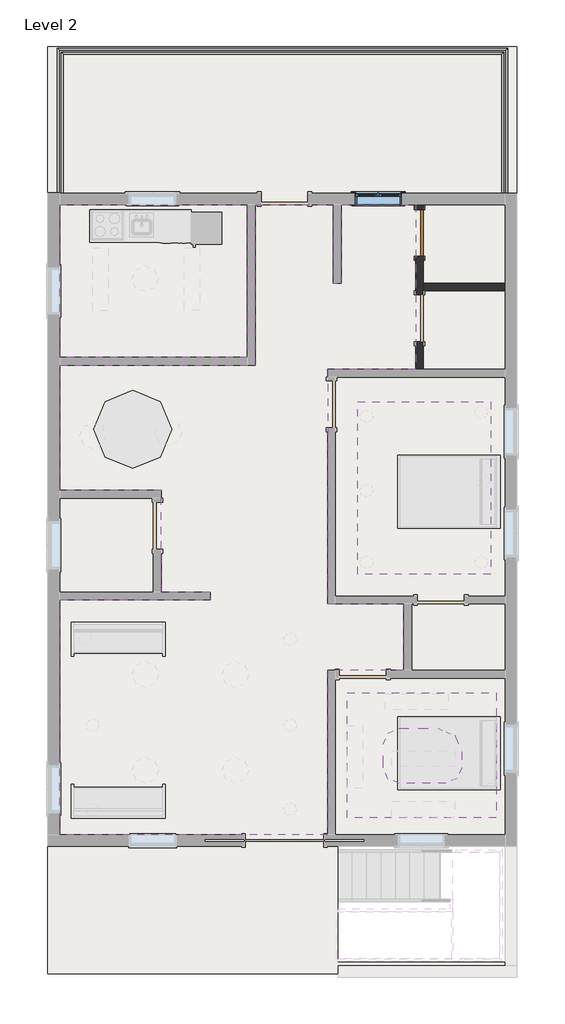
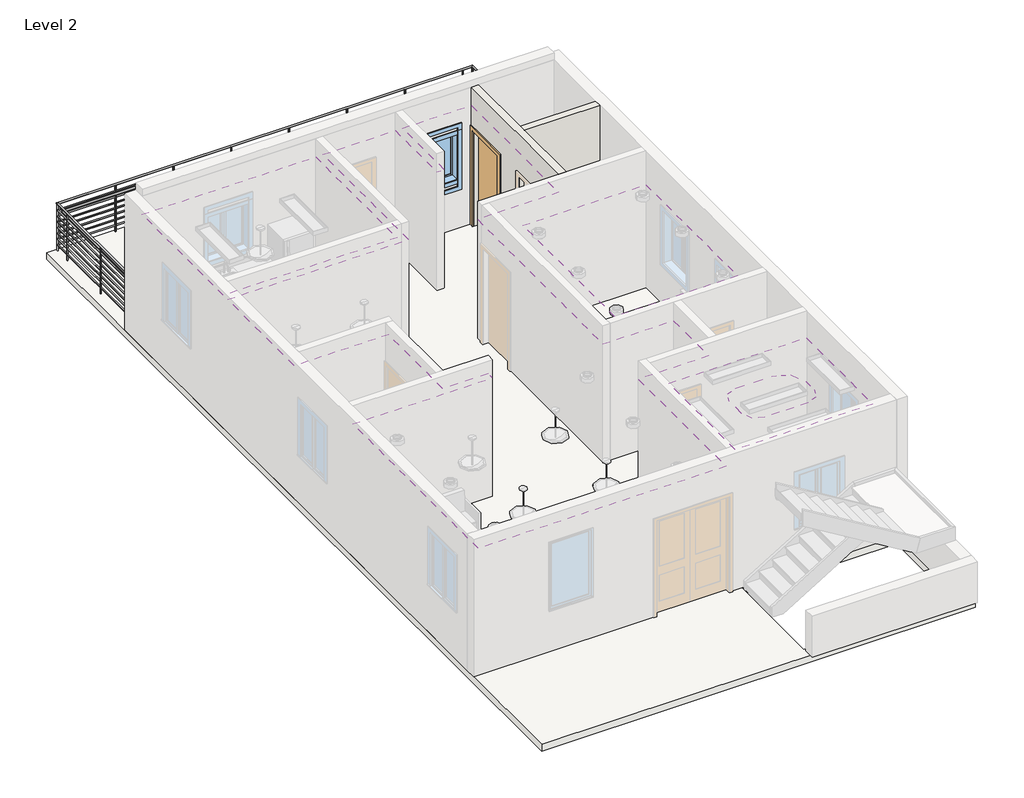
# One storey, part 2 of 3: 7 coverings, 2 walls, 2 windows, 1 door, 1 railing, 1 slab.
"""IFC4 building model written with IfcOpenShell, lengths in millimetres."""

from ifc_helpers import new_model, si_unit, point, frame, frame_2d, origin, place, context, project, spatial, polyline, circle_curve, ellipse_curve, trimmed, segment, composite_curve, outline, extrude, faceted_brep, transform, mapped, element, save
from ifc_brep_helpers import plane_surface, cylinder_surface, advanced_brep
from components import single_flush_single_door_686f89d2, window_419b5846

model = new_model("IFC4")

# Units and contexts
model_context = context("Model", 3, world=origin())
ifc_project = project(units=[si_unit("LENGTHUNIT", "METRE", prefix="MILLI")], contexts=[model_context])

# Site, building, storey
site = spatial("IfcSite", under=ifc_project)
building = spatial("IfcBuilding", under=site)
storey = spatial("IfcBuildingStorey", under=building, Name="Level 2", Elevation=3200.4)

# Coverings
placement = place(None, origin())
element("IfcCovering", 1, ObjectType="design", at=placement, inside=storey, context=model_context, shape_type="SweptSolid", body=[
    extrude(outline(polyline([(-1441.8942717, 10130.0102367), (-1441.8942717, 6777.2102367), (-4032.6942717, 6777.2102367), (-4032.6942717, 10130.0102367), (-1441.8942717, 10130.0102367)]), holes=[composite_curve([segment(polyline([(-1961.8324971, 9831.2802454), (-3524.6942717, 9831.2802454)]), True, "CONTINUOUS"), segment(trimmed(circle_curve(frame_2d((-3524.6942717, 9628.0802454)), 203.2), [point((-3524.6942717, 9831.2802454))], [point((-3727.8942717, 9628.0802454))], True, "CARTESIAN"), True, "CONTINUOUS"), segment(polyline([(-3727.8942717, 9628.0802454), (-3727.8942717, 7367.4802454)]), True, "CONTINUOUS"), segment(trimmed(circle_curve(frame_2d((-3397.6942717, 7367.4802454)), 330.2), [point((-3727.8942717, 7367.4802454))], [point((-3397.6942717, 7037.2802454))], True, "CARTESIAN"), True, "CONTINUOUS"), segment(polyline([(-3397.6942717, 7037.2802454), (-2178.4942717, 7037.2802454)]), True, "CONTINUOUS"), segment(trimmed(circle_curve(frame_2d((-2178.4942717, 7469.0802454)), 431.8), [point((-2178.4942717, 7037.2802454))], [point((-1746.6942717, 7469.0802454))], True, "CARTESIAN"), True, "CONTINUOUS"), segment(polyline([(-1746.6942717, 7469.0802454), (-1746.6942717, 9616.14202)]), True, "CONTINUOUS"), segment(trimmed(circle_curve(frame_2d((-1961.8324971, 9616.14202)), 215.1382254), [point((-1746.6942717, 9616.14202))], [point((-1961.8324971, 9831.2802454))], True, "CARTESIAN"), True, "CONTINUOUS")], self_intersect=False)]), frame((0.0, 0.0, 5892.8), z_axis=(0.0, 0.0, 1.0), x_axis=(1.0, 0.0, 0.0)), (0.0, 0.0, 1.0), 50.8),
])
element("IfcCovering", 2, ObjectType="design", at=placement, inside=storey, context=model_context, shape_type="SweptSolid", body=[
    extrude(outline(polyline([(-1336.1469547, 4466.8667258), (-1336.1469547, 2028.4667258), (-4231.7469547, 2028.4667258), (-4231.7469547, 4466.8667258), (-1336.1469547, 4466.8667258)]), holes=[polyline([(-1663.4737397, 4144.2687658), (-3949.4737397, 4144.2687658), (-3949.4737397, 2315.4687658), (-1663.4737397, 2315.4687658), (-1663.4737397, 4144.2687658)])]), frame((0.0, 0.0, 5880.0205268), z_axis=(0.0, 0.0, 1.0), x_axis=(1.0, 0.0, 0.0)), (0.0, 0.0, 1.0), 50.8),
])
element("IfcCovering", 3, ObjectType="inner", at=placement, inside=storey, context=model_context, shape_type="SweptSolid", body=[
    extrude(outline(composite_curve([segment(trimmed(circle_curve(frame_2d((-2465.984708, 3312.1230358)), 457.2), [point((-2465.984708, 3769.3230358))], [point((-2008.784708, 3312.1230358))], False, "CARTESIAN"), True, "CONTINUOUS"), segment(polyline([(-2008.784708, 3312.1230358), (-2008.784708, 3007.3230358)]), True, "CONTINUOUS"), segment(trimmed(circle_curve(frame_2d((-2313.584708, 3007.3230358)), 304.8), [point((-2008.784708, 3007.3230358))], [point((-2313.584708, 2702.5230358))], False, "CARTESIAN"), True, "CONTINUOUS"), segment(polyline([(-2313.584708, 2702.5230358), (-3227.984708, 2702.5230358)]), True, "CONTINUOUS"), segment(trimmed(circle_curve(frame_2d((-3227.984708, 3007.3230358)), 304.8), [point((-3227.984708, 2702.5230358))], [point((-3532.784708, 3007.3230358))], False, "CARTESIAN"), True, "CONTINUOUS"), segment(polyline([(-3532.784708, 3007.3230358), (-3532.784708, 3464.5230358)]), True, "CONTINUOUS"), segment(trimmed(circle_curve(frame_2d((-3227.984708, 3464.5230358)), 304.8), [point((-3532.784708, 3464.5230358))], [point((-3227.984708, 3769.3230358))], False, "CARTESIAN"), True, "CONTINUOUS"), segment(polyline([(-3227.984708, 3769.3230358), (-2465.984708, 3769.3230358)]), True, "CONTINUOUS")], self_intersect=False)), frame((0.0, 0.0, 5842.0), z_axis=(0.0, 0.0, 1.0), x_axis=(1.0, 0.0, 0.0)), (0.0, 0.0, 1.0), 50.8),
])
element("IfcCovering", 4, ObjectType="inner", at=placement, inside=storey, context=model_context, shape_type="SweptSolid", body=[
    extrude(outline(polyline([(-4619.1572065, 4901.2206867), (-4619.1572065, 1700.8206867), (-9838.8572065, 1700.8206867), (-9838.8572065, 6272.8206867), (-6905.1572065, 6272.8206867), (-6905.1572065, 6425.2206867), (-7857.6572065, 6425.2206867), (-7857.6572065, 8406.4206867), (-9838.8572065, 8406.4206867), (-9838.8572065, 10844.8206867), (-6028.8572065, 10844.8206867), (-6028.8572065, 13969.0206867), (-4504.8572065, 13969.0206867), (-4504.8572065, 12445.0206867), (-4352.4572065, 12445.0206867), (-4352.4572065, 13969.0206867), (-2904.6572065, 13969.0206867), (-2904.6572065, 10768.6206867), (-4619.1572065, 10768.6206867), (-4619.1572065, 6196.6206867), (-3133.2572065, 6196.6206867), (-3133.2572065, 4901.2206867), (-4619.1572065, 4901.2206867)])), frame((0.0, 0.0, 5842.0), z_axis=(0.0, 0.0, 1.0), x_axis=(1.0, 0.0, 0.0)), (0.0, 0.0, 1.0), 50.8),
])
element("IfcCovering", 5, ObjectType="inner", at=placement, inside=storey, context=model_context, shape_type="SweptSolid", body=[
    extrude(outline(polyline([(-4619.1572065, 4901.2206867), (-4619.1572065, 1700.8206867), (-9838.8572065, 1700.8206867), (-9838.8572065, 6272.8206867), (-6905.1572065, 6272.8206867), (-6905.1572065, 6425.2206867), (-7857.6572065, 6425.2206867), (-7857.6572065, 8406.4206867), (-9838.8572065, 8406.4206867), (-9838.8572065, 10844.8206867), (-6028.8572065, 10844.8206867), (-6028.8572065, 13969.0206867), (-4504.8572065, 13969.0206867), (-4504.8572065, 12445.0206867), (-4352.4572065, 12445.0206867), (-4352.4572065, 13969.0206867), (-2904.6572065, 13969.0206867), (-2904.6572065, 10768.6206867), (-4619.1572065, 10768.6206867), (-4619.1572065, 6196.6206867), (-3133.2572065, 6196.6206867), (-3133.2572065, 4901.2206867), (-4619.1572065, 4901.2206867)])), frame((0.0, 0.0, 5842.0), z_axis=(0.0, 0.0, 1.0), x_axis=(1.0, 0.0, 0.0)), (0.0, 0.0, 1.0), 50.8),
])
element("IfcCovering", 6, ObjectType="inner", at=placement, inside=storey, context=model_context, shape_type="SweptSolid", body=[
    extrude(outline(polyline([(-9838.8572065, 13969.0206867), (-6181.2572065, 13969.0206867), (-6181.2572065, 10997.2206867), (-9838.8572065, 10997.2206867), (-9838.8572065, 13969.0206867)])), frame((0.0, 0.0, 5842.0), z_axis=(0.0, 0.0, 1.0), x_axis=(1.0, 0.0, 0.0)), (0.0, 0.0, 1.0), 50.8),
])
element("IfcCovering", 7, ObjectType="inner", at=placement, inside=storey, context=model_context, shape_type="SweptSolid", body=[
    extrude(outline(polyline([(-9838.8572065, 13969.0206867), (-6181.2572065, 13969.0206867), (-6181.2572065, 10997.2206867), (-9838.8572065, 10997.2206867), (-9838.8572065, 13969.0206867)])), frame((0.0, 0.0, 5842.0), z_axis=(0.0, 0.0, 1.0), x_axis=(1.0, 0.0, 0.0)), (0.0, 0.0, 1.0), 50.8),
])

# Door
single_flush_single_door_shape = single_flush_single_door_686f89d2(model_context)
element("IfcDoor", 8, ObjectType="Single-Flush : single door", at=placement, inside=storey, context=model_context, shape_type="MappedRepresentation", body=[
    mapped(single_flush_single_door_shape, transform((-2828.4572065, 13422.9206867, 3200.4), x_axis=(0.0, 1.0, 0.0), y_axis=(-1.0, 0.0, 0.0), z_axis=(0.0, 0.0, 1.0))),
])

# Railing
element("IfcRailing", 9, ObjectType="Guardrail - Pipe", at=placement, inside=storey, context=model_context, shape_type="SolidModel", body=[
    advanced_brep(
    [(-9769.0072065, 14210.3206867, 4095.75), (-9807.1072065, 14210.3206867, 4095.75), (-9769.0072065, 16909.0706867, 4095.75), (-9807.1072065, 16947.1706867, 4095.75), (-1221.9072065, 16909.0706867, 4095.75), (-1183.8072065, 16947.1706867, 4095.75), (-1221.9072065, 14210.3206867, 4095.75), (-1183.8072065, 14210.3206867, 4095.75)],
    [
        (0, 1, circle_curve(frame((-9788.0572065, 14210.3206867, 4095.75), z_axis=(0.0, -1.0, 0.0), x_axis=(-1.0, 0.0, 0.0)), 19.05)),
        (1, 0, circle_curve(frame((-9788.0572065, 14210.3206867, 4095.75), z_axis=(0.0, -1.0, 0.0), x_axis=(-1.0, 0.0, 0.0)), 19.05)),
        (0, 2),
        (2, 3, ellipse_curve(frame((-9788.0572065, 16928.1206867, 4095.75), z_axis=(-0.7071067811865475, -0.7071067811865475, 0.0), x_axis=(0.7071067811865474, -0.7071067811865476, 0.0)), 26.9407684, 19.05)),
        (3, 1),
        (3, 2, ellipse_curve(frame((-9788.0572065, 16928.1206867, 4095.75), z_axis=(-0.7071067811865475, -0.7071067811865475, 0.0), x_axis=(0.7071067811865474, -0.7071067811865476, 0.0)), 26.9407684, 19.05)),
        (2, 4),
        (4, 5, ellipse_curve(frame((-1202.8572065, 16928.1206867, 4095.75), z_axis=(-0.7071067811865475, 0.7071067811865475, 0.0), x_axis=(-0.7071067811865476, -0.7071067811865474, 0.0)), 26.9407684, 19.05)),
        (5, 3),
        (5, 4, ellipse_curve(frame((-1202.8572065, 16928.1206867, 4095.75), z_axis=(-0.7071067811865475, 0.7071067811865475, 0.0), x_axis=(-0.7071067811865476, -0.7071067811865474, 0.0)), 26.9407684, 19.05)),
        (6, 7, circle_curve(frame((-1202.8572065, 14210.3206867, 4095.75), z_axis=(0.0, -1.0, 0.0), x_axis=(1.0, 0.0, 0.0)), 19.05)),
        (7, 6, circle_curve(frame((-1202.8572065, 14210.3206867, 4095.75), z_axis=(0.0, -1.0, 0.0), x_axis=(1.0, 0.0, 0.0)), 19.05)),
        (4, 6),
        (7, 5),
    ],
    [
        plane_surface(frame((-9788.0572065, 14210.3206867, 4114.8), z_axis=(0.0, -1.0, 0.0), x_axis=(0.0, 0.0, 1.0))),
        cylinder_surface(frame((-9788.0572065, 14210.3206867, 4095.75), z_axis=(0.0, -1.0, 0.0), x_axis=(-1.0, 0.0, 0.0)), 19.05),
        cylinder_surface(frame((-9788.0572065, 16928.1206867, 4095.75), z_axis=(-1.0, 0.0, 0.0), x_axis=(0.0, 1.0, 0.0)), 19.05),
        plane_surface(frame((-1202.8572065, 14210.3206867, 4114.8), z_axis=(0.0, -1.0, 0.0), x_axis=(0.0, 0.0, -1.0))),
        cylinder_surface(frame((-1202.8572065, 16928.1206867, 4095.75), z_axis=(0.0, 1.0, 0.0), x_axis=(1.0, 0.0, 0.0)), 19.05),
    ],
    [
        (0, [[1, 2]]),
        (1, [[-1, 3, 4, 5]]),
        (1, [[-2, -5, 6, -3]]),
        (2, [[-4, 7, 8, 9]]),
        (2, [[-6, -9, 10, -7]]),
        (3, [[11, 12]]),
        (4, [[-8, 13, -12, 14]]),
        (4, [[-10, -14, -11, -13]]),
    ],
),
    advanced_brep(
    [(-9845.2072065, 14210.3206867, 4248.15), (-9883.3072065, 14210.3206867, 4248.15), (-9845.2072065, 16985.2706867, 4248.15), (-9883.3072065, 17023.3706867, 4248.15), (-1145.7072065, 16985.2706867, 4248.15), (-1107.6072065, 17023.3706867, 4248.15), (-1145.7072065, 14210.3206867, 4248.15), (-1107.6072065, 14210.3206867, 4248.15)],
    [
        (0, 1, circle_curve(frame((-9864.2572065, 14210.3206867, 4248.15), z_axis=(0.0, -1.0, 0.0), x_axis=(-1.0, 0.0, 0.0)), 19.05)),
        (1, 0, circle_curve(frame((-9864.2572065, 14210.3206867, 4248.15), z_axis=(0.0, -1.0, 0.0), x_axis=(-1.0, 0.0, 0.0)), 19.05)),
        (0, 2),
        (2, 3, ellipse_curve(frame((-9864.2572065, 17004.3206867, 4248.15), z_axis=(-0.7071067811865475, -0.7071067811865475, 0.0), x_axis=(0.7071067811865474, -0.7071067811865476, 0.0)), 26.9407684, 19.05)),
        (3, 1),
        (3, 2, ellipse_curve(frame((-9864.2572065, 17004.3206867, 4248.15), z_axis=(-0.7071067811865475, -0.7071067811865475, 0.0), x_axis=(0.7071067811865474, -0.7071067811865476, 0.0)), 26.9407684, 19.05)),
        (2, 4),
        (4, 5, ellipse_curve(frame((-1126.6572065, 17004.3206867, 4248.15), z_axis=(-0.7071067811865475, 0.7071067811865475, 0.0), x_axis=(-0.7071067811865476, -0.7071067811865474, 0.0)), 26.9407684, 19.05)),
        (5, 3),
        (5, 4, ellipse_curve(frame((-1126.6572065, 17004.3206867, 4248.15), z_axis=(-0.7071067811865475, 0.7071067811865475, 0.0), x_axis=(-0.7071067811865476, -0.7071067811865474, 0.0)), 26.9407684, 19.05)),
        (6, 7, circle_curve(frame((-1126.6572065, 14210.3206867, 4248.15), z_axis=(0.0, -1.0, 0.0), x_axis=(1.0, 0.0, 0.0)), 19.05)),
        (7, 6, circle_curve(frame((-1126.6572065, 14210.3206867, 4248.15), z_axis=(0.0, -1.0, 0.0), x_axis=(1.0, 0.0, 0.0)), 19.05)),
        (4, 6),
        (7, 5),
    ],
    [
        plane_surface(frame((-9864.2572065, 14210.3206867, 4267.2), z_axis=(0.0, -1.0, 0.0), x_axis=(0.0, 0.0, 1.0))),
        cylinder_surface(frame((-9864.2572065, 14210.3206867, 4248.15), z_axis=(0.0, -1.0, 0.0), x_axis=(-1.0, 0.0, 0.0)), 19.05),
        cylinder_surface(frame((-9864.2572065, 17004.3206867, 4248.15), z_axis=(-1.0, 0.0, 0.0), x_axis=(0.0, 1.0, 0.0)), 19.05),
        plane_surface(frame((-1126.6572065, 14210.3206867, 4267.2), z_axis=(0.0, -1.0, 0.0), x_axis=(0.0, 0.0, -1.0))),
        cylinder_surface(frame((-1126.6572065, 17004.3206867, 4248.15), z_axis=(0.0, 1.0, 0.0), x_axis=(1.0, 0.0, 0.0)), 19.05),
    ],
    [
        (0, [[1, 2]]),
        (1, [[-1, 3, 4, 5]]),
        (1, [[-2, -5, 6, -3]]),
        (2, [[-4, 7, 8, 9]]),
        (2, [[-6, -9, 10, -7]]),
        (3, [[11, 12]]),
        (4, [[-8, 13, -12, 14]]),
        (4, [[-10, -14, -11, -13]]),
    ],
),
    advanced_brep(
    [(-9851.5572065, 14210.3206867, 4102.1), (-9876.9572065, 14210.3206867, 4102.1), (-9876.9572065, 17017.0206867, 4102.1), (-9851.5572065, 16991.6206867, 4102.1), (-1113.9572065, 17017.0206867, 4102.1), (-1139.3572065, 16991.6206867, 4102.1), (-1139.3572065, 14210.3206867, 4102.1), (-1113.9572065, 14210.3206867, 4102.1)],
    [
        (0, 1, circle_curve(frame((-9864.2572065, 14210.3206867, 4102.1), z_axis=(0.0, -1.0, 0.0), x_axis=(-1.0, 0.0, 0.0)), 12.7)),
        (1, 0, circle_curve(frame((-9864.2572065, 14210.3206867, 4102.1), z_axis=(0.0, -1.0, 0.0), x_axis=(-1.0, 0.0, 0.0)), 12.7)),
        (1, 2),
        (2, 3, ellipse_curve(frame((-9864.2572065, 17004.3206867, 4102.1), z_axis=(-0.7071067811865475, -0.7071067811865475, 0.0), x_axis=(0.7071067811865474, -0.7071067811865476, 0.0)), 17.9605122, 12.7)),
        (3, 0),
        (3, 2, ellipse_curve(frame((-9864.2572065, 17004.3206867, 4102.1), z_axis=(-0.7071067811865475, -0.7071067811865475, 0.0), x_axis=(0.7071067811865474, -0.7071067811865476, 0.0)), 17.9605122, 12.7)),
        (2, 4),
        (4, 5, ellipse_curve(frame((-1126.6572065, 17004.3206867, 4102.1), z_axis=(-0.7071067811865475, 0.7071067811865475, 0.0), x_axis=(-0.7071067811865476, -0.7071067811865474, 0.0)), 17.9605122, 12.7)),
        (5, 3),
        (5, 4, ellipse_curve(frame((-1126.6572065, 17004.3206867, 4102.1), z_axis=(-0.7071067811865475, 0.7071067811865475, 0.0), x_axis=(-0.7071067811865476, -0.7071067811865474, 0.0)), 17.9605122, 12.7)),
        (6, 7, circle_curve(frame((-1126.6572065, 14210.3206867, 4102.1), z_axis=(0.0, -1.0, 0.0), x_axis=(1.0, 0.0, 0.0)), 12.7)),
        (7, 6, circle_curve(frame((-1126.6572065, 14210.3206867, 4102.1), z_axis=(0.0, -1.0, 0.0), x_axis=(1.0, 0.0, 0.0)), 12.7)),
        (4, 7),
        (6, 5),
    ],
    [
        plane_surface(frame((-9864.2572065, 14210.3206867, 4114.8), z_axis=(0.0, -1.0, 0.0), x_axis=(0.0, 0.0, 1.0))),
        cylinder_surface(frame((-9864.2572065, 14210.3206867, 4102.1), z_axis=(0.0, -1.0, 0.0), x_axis=(-1.0, 0.0, 0.0)), 12.7),
        cylinder_surface(frame((-9864.2572065, 17004.3206867, 4102.1), z_axis=(-1.0, 0.0, 0.0), x_axis=(0.0, 1.0, 0.0)), 12.7),
        plane_surface(frame((-1126.6572065, 14210.3206867, 4114.8), z_axis=(0.0, -1.0, 0.0), x_axis=(0.0, 0.0, -1.0))),
        cylinder_surface(frame((-1126.6572065, 17004.3206867, 4102.1), z_axis=(0.0, 1.0, 0.0), x_axis=(1.0, 0.0, 0.0)), 12.7),
    ],
    [
        (0, [[1, 2]]),
        (1, [[-2, 3, 4, 5]]),
        (1, [[-1, -5, 6, -3]]),
        (2, [[-4, 7, 8, 9]]),
        (2, [[-6, -9, 10, -7]]),
        (3, [[11, 12]]),
        (4, [[-8, 13, -11, 14]]),
        (4, [[-10, -14, -12, -13]]),
    ],
),
    advanced_brep(
    [(-9851.5572065, 14210.3206867, 3975.1), (-9876.9572065, 14210.3206867, 3975.1), (-9876.9572065, 17017.0206867, 3975.1), (-9851.5572065, 16991.6206867, 3975.1), (-1113.9572065, 17017.0206867, 3975.1), (-1139.3572065, 16991.6206867, 3975.1), (-1139.3572065, 14210.3206867, 3975.1), (-1113.9572065, 14210.3206867, 3975.1)],
    [
        (0, 1, circle_curve(frame((-9864.2572065, 14210.3206867, 3975.1), z_axis=(0.0, -1.0, 0.0), x_axis=(-1.0, 0.0, 0.0)), 12.7)),
        (1, 0, circle_curve(frame((-9864.2572065, 14210.3206867, 3975.1), z_axis=(0.0, -1.0, 0.0), x_axis=(-1.0, 0.0, 0.0)), 12.7)),
        (1, 2),
        (2, 3, ellipse_curve(frame((-9864.2572065, 17004.3206867, 3975.1), z_axis=(-0.7071067811865475, -0.7071067811865475, 0.0), x_axis=(0.7071067811865474, -0.7071067811865476, 0.0)), 17.9605122, 12.7)),
        (3, 0),
        (3, 2, ellipse_curve(frame((-9864.2572065, 17004.3206867, 3975.1), z_axis=(-0.7071067811865475, -0.7071067811865475, 0.0), x_axis=(0.7071067811865474, -0.7071067811865476, 0.0)), 17.9605122, 12.7)),
        (2, 4),
        (4, 5, ellipse_curve(frame((-1126.6572065, 17004.3206867, 3975.1), z_axis=(-0.7071067811865475, 0.7071067811865475, 0.0), x_axis=(-0.7071067811865476, -0.7071067811865474, 0.0)), 17.9605122, 12.7)),
        (5, 3),
        (5, 4, ellipse_curve(frame((-1126.6572065, 17004.3206867, 3975.1), z_axis=(-0.7071067811865475, 0.7071067811865475, 0.0), x_axis=(-0.7071067811865476, -0.7071067811865474, 0.0)), 17.9605122, 12.7)),
        (6, 7, circle_curve(frame((-1126.6572065, 14210.3206867, 3975.1), z_axis=(0.0, -1.0, 0.0), x_axis=(1.0, 0.0, 0.0)), 12.7)),
        (7, 6, circle_curve(frame((-1126.6572065, 14210.3206867, 3975.1), z_axis=(0.0, -1.0, 0.0), x_axis=(1.0, 0.0, 0.0)), 12.7)),
        (4, 7),
        (6, 5),
    ],
    [
        plane_surface(frame((-9864.2572065, 14210.3206867, 3987.8), z_axis=(0.0, -1.0, 0.0), x_axis=(0.0, 0.0, 1.0))),
        cylinder_surface(frame((-9864.2572065, 14210.3206867, 3975.1), z_axis=(0.0, -1.0, 0.0), x_axis=(-1.0, 0.0, 0.0)), 12.7),
        cylinder_surface(frame((-9864.2572065, 17004.3206867, 3975.1), z_axis=(-1.0, 0.0, 0.0), x_axis=(0.0, 1.0, 0.0)), 12.7),
        plane_surface(frame((-1126.6572065, 14210.3206867, 3987.8), z_axis=(0.0, -1.0, 0.0), x_axis=(0.0, 0.0, -1.0))),
        cylinder_surface(frame((-1126.6572065, 17004.3206867, 3975.1), z_axis=(0.0, 1.0, 0.0), x_axis=(1.0, 0.0, 0.0)), 12.7),
    ],
    [
        (0, [[1, 2]]),
        (1, [[-2, 3, 4, 5]]),
        (1, [[-1, -5, 6, -3]]),
        (2, [[-4, 7, 8, 9]]),
        (2, [[-6, -9, 10, -7]]),
        (3, [[11, 12]]),
        (4, [[-8, 13, -11, 14]]),
        (4, [[-10, -14, -12, -13]]),
    ],
),
    advanced_brep(
    [(-9851.5572065, 14210.3206867, 3848.1), (-9876.9572065, 14210.3206867, 3848.1), (-9876.9572065, 17017.0206867, 3848.1), (-9851.5572065, 16991.6206867, 3848.1), (-1113.9572065, 17017.0206867, 3848.1), (-1139.3572065, 16991.6206867, 3848.1), (-1139.3572065, 14210.3206867, 3848.1), (-1113.9572065, 14210.3206867, 3848.1)],
    [
        (0, 1, circle_curve(frame((-9864.2572065, 14210.3206867, 3848.1), z_axis=(0.0, -1.0, 0.0), x_axis=(-1.0, 0.0, 0.0)), 12.7)),
        (1, 0, circle_curve(frame((-9864.2572065, 14210.3206867, 3848.1), z_axis=(0.0, -1.0, 0.0), x_axis=(-1.0, 0.0, 0.0)), 12.7)),
        (1, 2),
        (2, 3, ellipse_curve(frame((-9864.2572065, 17004.3206867, 3848.1), z_axis=(-0.7071067811865475, -0.7071067811865475, 0.0), x_axis=(0.7071067811865474, -0.7071067811865476, 0.0)), 17.9605122, 12.7)),
        (3, 0),
        (3, 2, ellipse_curve(frame((-9864.2572065, 17004.3206867, 3848.1), z_axis=(-0.7071067811865475, -0.7071067811865475, 0.0), x_axis=(0.7071067811865474, -0.7071067811865476, 0.0)), 17.9605122, 12.7)),
        (2, 4),
        (4, 5, ellipse_curve(frame((-1126.6572065, 17004.3206867, 3848.1), z_axis=(-0.7071067811865475, 0.7071067811865475, 0.0), x_axis=(-0.7071067811865476, -0.7071067811865474, 0.0)), 17.9605122, 12.7)),
        (5, 3),
        (5, 4, ellipse_curve(frame((-1126.6572065, 17004.3206867, 3848.1), z_axis=(-0.7071067811865475, 0.7071067811865475, 0.0), x_axis=(-0.7071067811865476, -0.7071067811865474, 0.0)), 17.9605122, 12.7)),
        (6, 7, circle_curve(frame((-1126.6572065, 14210.3206867, 3848.1), z_axis=(0.0, -1.0, 0.0), x_axis=(1.0, 0.0, 0.0)), 12.7)),
        (7, 6, circle_curve(frame((-1126.6572065, 14210.3206867, 3848.1), z_axis=(0.0, -1.0, 0.0), x_axis=(1.0, 0.0, 0.0)), 12.7)),
        (4, 7),
        (6, 5),
    ],
    [
        plane_surface(frame((-9864.2572065, 14210.3206867, 3860.8), z_axis=(0.0, -1.0, 0.0), x_axis=(0.0, 0.0, 1.0))),
        cylinder_surface(frame((-9864.2572065, 14210.3206867, 3848.1), z_axis=(0.0, -1.0, 0.0), x_axis=(-1.0, 0.0, 0.0)), 12.7),
        cylinder_surface(frame((-9864.2572065, 17004.3206867, 3848.1), z_axis=(-1.0, 0.0, 0.0), x_axis=(0.0, 1.0, 0.0)), 12.7),
        plane_surface(frame((-1126.6572065, 14210.3206867, 3860.8), z_axis=(0.0, -1.0, 0.0), x_axis=(0.0, 0.0, -1.0))),
        cylinder_surface(frame((-1126.6572065, 17004.3206867, 3848.1), z_axis=(0.0, 1.0, 0.0), x_axis=(1.0, 0.0, 0.0)), 12.7),
    ],
    [
        (0, [[1, 2]]),
        (1, [[-2, 3, 4, 5]]),
        (1, [[-1, -5, 6, -3]]),
        (2, [[-4, 7, 8, 9]]),
        (2, [[-6, -9, 10, -7]]),
        (3, [[11, 12]]),
        (4, [[-8, 13, -11, 14]]),
        (4, [[-10, -14, -12, -13]]),
    ],
),
    advanced_brep(
    [(-9851.5572065, 14210.3206867, 3721.1), (-9876.9572065, 14210.3206867, 3721.1), (-9876.9572065, 17017.0206867, 3721.1), (-9851.5572065, 16991.6206867, 3721.1), (-1113.9572065, 17017.0206867, 3721.1), (-1139.3572065, 16991.6206867, 3721.1), (-1139.3572065, 14210.3206867, 3721.1), (-1113.9572065, 14210.3206867, 3721.1)],
    [
        (0, 1, circle_curve(frame((-9864.2572065, 14210.3206867, 3721.1), z_axis=(0.0, -1.0, 0.0), x_axis=(-1.0, 0.0, 0.0)), 12.7)),
        (1, 0, circle_curve(frame((-9864.2572065, 14210.3206867, 3721.1), z_axis=(0.0, -1.0, 0.0), x_axis=(-1.0, 0.0, 0.0)), 12.7)),
        (1, 2),
        (2, 3, ellipse_curve(frame((-9864.2572065, 17004.3206867, 3721.1), z_axis=(-0.7071067811865475, -0.7071067811865475, 0.0), x_axis=(0.7071067811865474, -0.7071067811865476, 0.0)), 17.9605122, 12.7)),
        (3, 0),
        (3, 2, ellipse_curve(frame((-9864.2572065, 17004.3206867, 3721.1), z_axis=(-0.7071067811865475, -0.7071067811865475, 0.0), x_axis=(0.7071067811865474, -0.7071067811865476, 0.0)), 17.9605122, 12.7)),
        (2, 4),
        (4, 5, ellipse_curve(frame((-1126.6572065, 17004.3206867, 3721.1), z_axis=(-0.7071067811865475, 0.7071067811865475, 0.0), x_axis=(-0.7071067811865476, -0.7071067811865474, 0.0)), 17.9605122, 12.7)),
        (5, 3),
        (5, 4, ellipse_curve(frame((-1126.6572065, 17004.3206867, 3721.1), z_axis=(-0.7071067811865475, 0.7071067811865475, 0.0), x_axis=(-0.7071067811865476, -0.7071067811865474, 0.0)), 17.9605122, 12.7)),
        (6, 7, circle_curve(frame((-1126.6572065, 14210.3206867, 3721.1), z_axis=(0.0, -1.0, 0.0), x_axis=(1.0, 0.0, 0.0)), 12.7)),
        (7, 6, circle_curve(frame((-1126.6572065, 14210.3206867, 3721.1), z_axis=(0.0, -1.0, 0.0), x_axis=(1.0, 0.0, 0.0)), 12.7)),
        (4, 7),
        (6, 5),
    ],
    [
        plane_surface(frame((-9864.2572065, 14210.3206867, 3733.8), z_axis=(0.0, -1.0, 0.0), x_axis=(0.0, 0.0, 1.0))),
        cylinder_surface(frame((-9864.2572065, 14210.3206867, 3721.1), z_axis=(0.0, -1.0, 0.0), x_axis=(-1.0, 0.0, 0.0)), 12.7),
        cylinder_surface(frame((-9864.2572065, 17004.3206867, 3721.1), z_axis=(-1.0, 0.0, 0.0), x_axis=(0.0, 1.0, 0.0)), 12.7),
        plane_surface(frame((-1126.6572065, 14210.3206867, 3733.8), z_axis=(0.0, -1.0, 0.0), x_axis=(0.0, 0.0, -1.0))),
        cylinder_surface(frame((-1126.6572065, 17004.3206867, 3721.1), z_axis=(0.0, 1.0, 0.0), x_axis=(1.0, 0.0, 0.0)), 12.7),
    ],
    [
        (0, [[1, 2]]),
        (1, [[-2, 3, 4, 5]]),
        (1, [[-1, -5, 6, -3]]),
        (2, [[-4, 7, 8, 9]]),
        (2, [[-6, -9, 10, -7]]),
        (3, [[11, 12]]),
        (4, [[-8, 13, -11, 14]]),
        (4, [[-10, -14, -12, -13]]),
    ],
),
    advanced_brep(
    [(-9851.5572065, 14210.3206867, 3594.1), (-9876.9572065, 14210.3206867, 3594.1), (-9876.9572065, 17017.0206867, 3594.1), (-9851.5572065, 16991.6206867, 3594.1), (-1113.9572065, 17017.0206867, 3594.1), (-1139.3572065, 16991.6206867, 3594.1), (-1139.3572065, 14210.3206867, 3594.1), (-1113.9572065, 14210.3206867, 3594.1)],
    [
        (0, 1, circle_curve(frame((-9864.2572065, 14210.3206867, 3594.1), z_axis=(0.0, -1.0, 0.0), x_axis=(-1.0, 0.0, 0.0)), 12.7)),
        (1, 0, circle_curve(frame((-9864.2572065, 14210.3206867, 3594.1), z_axis=(0.0, -1.0, 0.0), x_axis=(-1.0, 0.0, 0.0)), 12.7)),
        (1, 2),
        (2, 3, ellipse_curve(frame((-9864.2572065, 17004.3206867, 3594.1), z_axis=(-0.7071067811865475, -0.7071067811865475, 0.0), x_axis=(0.7071067811865474, -0.7071067811865476, 0.0)), 17.9605122, 12.7)),
        (3, 0),
        (3, 2, ellipse_curve(frame((-9864.2572065, 17004.3206867, 3594.1), z_axis=(-0.7071067811865475, -0.7071067811865475, 0.0), x_axis=(0.7071067811865474, -0.7071067811865476, 0.0)), 17.9605122, 12.7)),
        (2, 4),
        (4, 5, ellipse_curve(frame((-1126.6572065, 17004.3206867, 3594.1), z_axis=(-0.7071067811865475, 0.7071067811865475, 0.0), x_axis=(-0.7071067811865476, -0.7071067811865474, 0.0)), 17.9605122, 12.7)),
        (5, 3),
        (5, 4, ellipse_curve(frame((-1126.6572065, 17004.3206867, 3594.1), z_axis=(-0.7071067811865475, 0.7071067811865475, 0.0), x_axis=(-0.7071067811865476, -0.7071067811865474, 0.0)), 17.9605122, 12.7)),
        (6, 7, circle_curve(frame((-1126.6572065, 14210.3206867, 3594.1), z_axis=(0.0, -1.0, 0.0), x_axis=(1.0, 0.0, 0.0)), 12.7)),
        (7, 6, circle_curve(frame((-1126.6572065, 14210.3206867, 3594.1), z_axis=(0.0, -1.0, 0.0), x_axis=(1.0, 0.0, 0.0)), 12.7)),
        (4, 7),
        (6, 5),
    ],
    [
        plane_surface(frame((-9864.2572065, 14210.3206867, 3606.8), z_axis=(0.0, -1.0, 0.0), x_axis=(0.0, 0.0, 1.0))),
        cylinder_surface(frame((-9864.2572065, 14210.3206867, 3594.1), z_axis=(0.0, -1.0, 0.0), x_axis=(-1.0, 0.0, 0.0)), 12.7),
        cylinder_surface(frame((-9864.2572065, 17004.3206867, 3594.1), z_axis=(-1.0, 0.0, 0.0), x_axis=(0.0, 1.0, 0.0)), 12.7),
        plane_surface(frame((-1126.6572065, 14210.3206867, 3606.8), z_axis=(0.0, -1.0, 0.0), x_axis=(0.0, 0.0, -1.0))),
        cylinder_surface(frame((-1126.6572065, 17004.3206867, 3594.1), z_axis=(0.0, 1.0, 0.0), x_axis=(1.0, 0.0, 0.0)), 12.7),
    ],
    [
        (0, [[1, 2]]),
        (1, [[-2, 3, 4, 5]]),
        (1, [[-1, -5, 6, -3]]),
        (2, [[-4, 7, 8, 9]]),
        (2, [[-6, -9, 10, -7]]),
        (3, [[11, 12]]),
        (4, [[-8, 13, -11, 14]]),
        (4, [[-10, -14, -12, -13]]),
    ],
),
    advanced_brep(
    [(-9851.5572065, 14210.3206867, 3467.1), (-9876.9572065, 14210.3206867, 3467.1), (-9876.9572065, 17017.0206867, 3467.1), (-9851.5572065, 16991.6206867, 3467.1), (-1113.9572065, 17017.0206867, 3467.1), (-1139.3572065, 16991.6206867, 3467.1), (-1139.3572065, 14210.3206867, 3467.1), (-1113.9572065, 14210.3206867, 3467.1)],
    [
        (0, 1, circle_curve(frame((-9864.2572065, 14210.3206867, 3467.1), z_axis=(0.0, -1.0, 0.0), x_axis=(-1.0, 0.0, 0.0)), 12.7)),
        (1, 0, circle_curve(frame((-9864.2572065, 14210.3206867, 3467.1), z_axis=(0.0, -1.0, 0.0), x_axis=(-1.0, 0.0, 0.0)), 12.7)),
        (1, 2),
        (2, 3, ellipse_curve(frame((-9864.2572065, 17004.3206867, 3467.1), z_axis=(-0.7071067811865475, -0.7071067811865475, 0.0), x_axis=(0.7071067811865474, -0.7071067811865476, 0.0)), 17.9605122, 12.7)),
        (3, 0),
        (3, 2, ellipse_curve(frame((-9864.2572065, 17004.3206867, 3467.1), z_axis=(-0.7071067811865475, -0.7071067811865475, 0.0), x_axis=(0.7071067811865474, -0.7071067811865476, 0.0)), 17.9605122, 12.7)),
        (2, 4),
        (4, 5, ellipse_curve(frame((-1126.6572065, 17004.3206867, 3467.1), z_axis=(-0.7071067811865475, 0.7071067811865475, 0.0), x_axis=(-0.7071067811865476, -0.7071067811865474, 0.0)), 17.9605122, 12.7)),
        (5, 3),
        (5, 4, ellipse_curve(frame((-1126.6572065, 17004.3206867, 3467.1), z_axis=(-0.7071067811865475, 0.7071067811865475, 0.0), x_axis=(-0.7071067811865476, -0.7071067811865474, 0.0)), 17.9605122, 12.7)),
        (6, 7, circle_curve(frame((-1126.6572065, 14210.3206867, 3467.1), z_axis=(0.0, -1.0, 0.0), x_axis=(1.0, 0.0, 0.0)), 12.7)),
        (7, 6, circle_curve(frame((-1126.6572065, 14210.3206867, 3467.1), z_axis=(0.0, -1.0, 0.0), x_axis=(1.0, 0.0, 0.0)), 12.7)),
        (4, 7),
        (6, 5),
    ],
    [
        plane_surface(frame((-9864.2572065, 14210.3206867, 3479.8), z_axis=(0.0, -1.0, 0.0), x_axis=(0.0, 0.0, 1.0))),
        cylinder_surface(frame((-9864.2572065, 14210.3206867, 3467.1), z_axis=(0.0, -1.0, 0.0), x_axis=(-1.0, 0.0, 0.0)), 12.7),
        cylinder_surface(frame((-9864.2572065, 17004.3206867, 3467.1), z_axis=(-1.0, 0.0, 0.0), x_axis=(0.0, 1.0, 0.0)), 12.7),
        plane_surface(frame((-1126.6572065, 14210.3206867, 3479.8), z_axis=(0.0, -1.0, 0.0), x_axis=(0.0, 0.0, -1.0))),
        cylinder_surface(frame((-1126.6572065, 17004.3206867, 3467.1), z_axis=(0.0, 1.0, 0.0), x_axis=(1.0, 0.0, 0.0)), 12.7),
    ],
    [
        (0, [[1, 2]]),
        (1, [[-2, 3, 4, 5]]),
        (1, [[-1, -5, 6, -3]]),
        (2, [[-4, 7, 8, 9]]),
        (2, [[-6, -9, 10, -7]]),
        (3, [[11, 12]]),
        (4, [[-8, 13, -11, 14]]),
        (4, [[-10, -14, -12, -13]]),
    ],
),
    advanced_brep(
    [(-9851.5572065, 14210.3206867, 3340.1), (-9876.9572065, 14210.3206867, 3340.1), (-9876.9572065, 17017.0206867, 3340.1), (-9851.5572065, 16991.6206867, 3340.1), (-1113.9572065, 17017.0206867, 3340.1), (-1139.3572065, 16991.6206867, 3340.1), (-1139.3572065, 14210.3206867, 3340.1), (-1113.9572065, 14210.3206867, 3340.1)],
    [
        (0, 1, circle_curve(frame((-9864.2572065, 14210.3206867, 3340.1), z_axis=(0.0, -1.0, 0.0), x_axis=(-1.0, 0.0, 0.0)), 12.7)),
        (1, 0, circle_curve(frame((-9864.2572065, 14210.3206867, 3340.1), z_axis=(0.0, -1.0, 0.0), x_axis=(-1.0, 0.0, 0.0)), 12.7)),
        (1, 2),
        (2, 3, ellipse_curve(frame((-9864.2572065, 17004.3206867, 3340.1), z_axis=(-0.7071067811865475, -0.7071067811865475, 0.0), x_axis=(0.7071067811865474, -0.7071067811865476, 0.0)), 17.9605122, 12.7)),
        (3, 0),
        (3, 2, ellipse_curve(frame((-9864.2572065, 17004.3206867, 3340.1), z_axis=(-0.7071067811865475, -0.7071067811865475, 0.0), x_axis=(0.7071067811865474, -0.7071067811865476, 0.0)), 17.9605122, 12.7)),
        (2, 4),
        (4, 5, ellipse_curve(frame((-1126.6572065, 17004.3206867, 3340.1), z_axis=(-0.7071067811865475, 0.7071067811865475, 0.0), x_axis=(-0.7071067811865476, -0.7071067811865474, 0.0)), 17.9605122, 12.7)),
        (5, 3),
        (5, 4, ellipse_curve(frame((-1126.6572065, 17004.3206867, 3340.1), z_axis=(-0.7071067811865475, 0.7071067811865475, 0.0), x_axis=(-0.7071067811865476, -0.7071067811865474, 0.0)), 17.9605122, 12.7)),
        (6, 7, circle_curve(frame((-1126.6572065, 14210.3206867, 3340.1), z_axis=(0.0, -1.0, 0.0), x_axis=(1.0, 0.0, 0.0)), 12.7)),
        (7, 6, circle_curve(frame((-1126.6572065, 14210.3206867, 3340.1), z_axis=(0.0, -1.0, 0.0), x_axis=(1.0, 0.0, 0.0)), 12.7)),
        (4, 7),
        (6, 5),
    ],
    [
        plane_surface(frame((-9864.2572065, 14210.3206867, 3352.8), z_axis=(0.0, -1.0, 0.0), x_axis=(0.0, 0.0, 1.0))),
        cylinder_surface(frame((-9864.2572065, 14210.3206867, 3340.1), z_axis=(0.0, -1.0, 0.0), x_axis=(-1.0, 0.0, 0.0)), 12.7),
        cylinder_surface(frame((-9864.2572065, 17004.3206867, 3340.1), z_axis=(-1.0, 0.0, 0.0), x_axis=(0.0, 1.0, 0.0)), 12.7),
        plane_surface(frame((-1126.6572065, 14210.3206867, 3352.8), z_axis=(0.0, -1.0, 0.0), x_axis=(0.0, 0.0, -1.0))),
        cylinder_surface(frame((-1126.6572065, 17004.3206867, 3340.1), z_axis=(0.0, 1.0, 0.0), x_axis=(1.0, 0.0, 0.0)), 12.7),
    ],
    [
        (0, [[1, 2]]),
        (1, [[-2, 3, 4, 5]]),
        (1, [[-1, -5, 6, -3]]),
        (2, [[-4, 7, 8, 9]]),
        (2, [[-6, -9, 10, -7]]),
        (3, [[11, 12]]),
        (4, [[-8, 13, -11, 14]]),
        (4, [[-10, -14, -12, -13]]),
    ],
),
    extrude(outline(composite_curve([segment(trimmed(circle_curve(frame_2d((-1126.6572065, 14565.9206867)), 12.7), [point((-1139.3572065, 14565.9206867))], [point((-1113.9572065, 14565.9206867))], False, "CARTESIAN"), True, "CONTINUOUS"), segment(trimmed(circle_curve(frame_2d((-1126.6572065, 14565.9206867)), 12.7), [point((-1113.9572065, 14565.9206867))], [point((-1139.3572065, 14565.9206867))], False, "CARTESIAN"), True, "CONTINUOUS")], self_intersect=False)), frame((0.0, 0.0, 3200.4), z_axis=(0.0, 0.0, 1.0), x_axis=(1.0, 0.0, 0.0)), (0.0, 0.0, 1.0), 1028.7),
    extrude(outline(composite_curve([segment(trimmed(circle_curve(frame_2d((-1126.6572065, 15785.1206867)), 12.7), [point((-1139.3572065, 15785.1206867))], [point((-1113.9572065, 15785.1206867))], False, "CARTESIAN"), True, "CONTINUOUS"), segment(trimmed(circle_curve(frame_2d((-1126.6572065, 15785.1206867)), 12.7), [point((-1113.9572065, 15785.1206867))], [point((-1139.3572065, 15785.1206867))], False, "CARTESIAN"), True, "CONTINUOUS")], self_intersect=False)), frame((0.0, 0.0, 3200.4), z_axis=(0.0, 0.0, 1.0), x_axis=(1.0, 0.0, 0.0)), (0.0, 0.0, 1.0), 1028.7),
    extrude(outline(composite_curve([segment(trimmed(circle_curve(frame_2d((-1329.8572065, 17004.3206867)), 12.7), [point((-1329.8572065, 16991.6206867))], [point((-1329.8572065, 17017.0206867))], False, "CARTESIAN"), True, "CONTINUOUS"), segment(trimmed(circle_curve(frame_2d((-1329.8572065, 17004.3206867)), 12.7), [point((-1329.8572065, 17017.0206867))], [point((-1329.8572065, 16991.6206867))], False, "CARTESIAN"), True, "CONTINUOUS")], self_intersect=False)), frame((0.0, 0.0, 3200.4), z_axis=(0.0, 0.0, 1.0), x_axis=(1.0, 0.0, 0.0)), (0.0, 0.0, 1.0), 1028.7),
    extrude(outline(composite_curve([segment(trimmed(circle_curve(frame_2d((-2549.0572065, 17004.3206867)), 12.7), [point((-2549.0572065, 16991.6206867))], [point((-2549.0572065, 17017.0206867))], False, "CARTESIAN"), True, "CONTINUOUS"), segment(trimmed(circle_curve(frame_2d((-2549.0572065, 17004.3206867)), 12.7), [point((-2549.0572065, 17017.0206867))], [point((-2549.0572065, 16991.6206867))], False, "CARTESIAN"), True, "CONTINUOUS")], self_intersect=False)), frame((0.0, 0.0, 3200.4), z_axis=(0.0, 0.0, 1.0), x_axis=(1.0, 0.0, 0.0)), (0.0, 0.0, 1.0), 1028.7),
    extrude(outline(composite_curve([segment(trimmed(circle_curve(frame_2d((-3768.2572065, 17004.3206867)), 12.7), [point((-3768.2572065, 16991.6206867))], [point((-3768.2572065, 17017.0206867))], False, "CARTESIAN"), True, "CONTINUOUS"), segment(trimmed(circle_curve(frame_2d((-3768.2572065, 17004.3206867)), 12.7), [point((-3768.2572065, 17017.0206867))], [point((-3768.2572065, 16991.6206867))], False, "CARTESIAN"), True, "CONTINUOUS")], self_intersect=False)), frame((0.0, 0.0, 3200.4), z_axis=(0.0, 0.0, 1.0), x_axis=(1.0, 0.0, 0.0)), (0.0, 0.0, 1.0), 1028.7),
    extrude(outline(composite_curve([segment(trimmed(circle_curve(frame_2d((-4987.4572065, 17004.3206867)), 12.7), [point((-4987.4572065, 16991.6206867))], [point((-4987.4572065, 17017.0206867))], False, "CARTESIAN"), True, "CONTINUOUS"), segment(trimmed(circle_curve(frame_2d((-4987.4572065, 17004.3206867)), 12.7), [point((-4987.4572065, 17017.0206867))], [point((-4987.4572065, 16991.6206867))], False, "CARTESIAN"), True, "CONTINUOUS")], self_intersect=False)), frame((0.0, 0.0, 3200.4), z_axis=(0.0, 0.0, 1.0), x_axis=(1.0, 0.0, 0.0)), (0.0, 0.0, 1.0), 1028.7),
    extrude(outline(composite_curve([segment(trimmed(circle_curve(frame_2d((-6206.6572065, 17004.3206867)), 12.7), [point((-6206.6572065, 16991.6206867))], [point((-6206.6572065, 17017.0206867))], False, "CARTESIAN"), True, "CONTINUOUS"), segment(trimmed(circle_curve(frame_2d((-6206.6572065, 17004.3206867)), 12.7), [point((-6206.6572065, 17017.0206867))], [point((-6206.6572065, 16991.6206867))], False, "CARTESIAN"), True, "CONTINUOUS")], self_intersect=False)), frame((0.0, 0.0, 3200.4), z_axis=(0.0, 0.0, 1.0), x_axis=(1.0, 0.0, 0.0)), (0.0, 0.0, 1.0), 1028.7),
    extrude(outline(composite_curve([segment(trimmed(circle_curve(frame_2d((-7425.8572065, 17004.3206867)), 12.7), [point((-7425.8572065, 16991.6206867))], [point((-7425.8572065, 17017.0206867))], False, "CARTESIAN"), True, "CONTINUOUS"), segment(trimmed(circle_curve(frame_2d((-7425.8572065, 17004.3206867)), 12.7), [point((-7425.8572065, 17017.0206867))], [point((-7425.8572065, 16991.6206867))], False, "CARTESIAN"), True, "CONTINUOUS")], self_intersect=False)), frame((0.0, 0.0, 3200.4), z_axis=(0.0, 0.0, 1.0), x_axis=(1.0, 0.0, 0.0)), (0.0, 0.0, 1.0), 1028.7),
    extrude(outline(composite_curve([segment(trimmed(circle_curve(frame_2d((-8645.0572065, 17004.3206867)), 12.7), [point((-8645.0572065, 16991.6206867))], [point((-8645.0572065, 17017.0206867))], False, "CARTESIAN"), True, "CONTINUOUS"), segment(trimmed(circle_curve(frame_2d((-8645.0572065, 17004.3206867)), 12.7), [point((-8645.0572065, 17017.0206867))], [point((-8645.0572065, 16991.6206867))], False, "CARTESIAN"), True, "CONTINUOUS")], self_intersect=False)), frame((0.0, 0.0, 3200.4), z_axis=(0.0, 0.0, 1.0), x_axis=(1.0, 0.0, 0.0)), (0.0, 0.0, 1.0), 1028.7),
    extrude(outline(composite_curve([segment(trimmed(circle_curve(frame_2d((-9864.2572065, 16648.7206867)), 12.7), [point((-9851.5572065, 16648.7206867))], [point((-9876.9572065, 16648.7206867))], False, "CARTESIAN"), True, "CONTINUOUS"), segment(trimmed(circle_curve(frame_2d((-9864.2572065, 16648.7206867)), 12.7), [point((-9876.9572065, 16648.7206867))], [point((-9851.5572065, 16648.7206867))], False, "CARTESIAN"), True, "CONTINUOUS")], self_intersect=False)), frame((0.0, 0.0, 3200.4), z_axis=(0.0, 0.0, 1.0), x_axis=(1.0, 0.0, 0.0)), (0.0, 0.0, 1.0), 1028.7),
    extrude(outline(composite_curve([segment(trimmed(circle_curve(frame_2d((-9864.2572065, 15429.5206867)), 12.7), [point((-9851.5572065, 15429.5206867))], [point((-9876.9572065, 15429.5206867))], False, "CARTESIAN"), True, "CONTINUOUS"), segment(trimmed(circle_curve(frame_2d((-9864.2572065, 15429.5206867)), 12.7), [point((-9876.9572065, 15429.5206867))], [point((-9851.5572065, 15429.5206867))], False, "CARTESIAN"), True, "CONTINUOUS")], self_intersect=False)), frame((0.0, 0.0, 3200.4), z_axis=(0.0, 0.0, 1.0), x_axis=(1.0, 0.0, 0.0)), (0.0, 0.0, 1.0), 1028.7),
    extrude(outline(composite_curve([segment(trimmed(circle_curve(frame_2d((-1126.6572065, 17004.3206867)), 12.7), [point((-1126.6572065, 16991.6206867))], [point((-1126.6572065, 17017.0206867))], False, "CARTESIAN"), True, "CONTINUOUS"), segment(trimmed(circle_curve(frame_2d((-1126.6572065, 17004.3206867)), 12.7), [point((-1126.6572065, 17017.0206867))], [point((-1126.6572065, 16991.6206867))], False, "CARTESIAN"), True, "CONTINUOUS")], self_intersect=False)), frame((0.0, 0.0, 3200.4), z_axis=(0.0, 0.0, 1.0), x_axis=(1.0, 0.0, 0.0)), (0.0, 0.0, 1.0), 1028.7),
    extrude(outline(composite_curve([segment(trimmed(circle_curve(frame_2d((-9864.2572065, 17004.3206867)), 12.7), [point((-9851.5572065, 17004.3206867))], [point((-9876.9572065, 17004.3206867))], False, "CARTESIAN"), True, "CONTINUOUS"), segment(trimmed(circle_curve(frame_2d((-9864.2572065, 17004.3206867)), 12.7), [point((-9876.9572065, 17004.3206867))], [point((-9851.5572065, 17004.3206867))], False, "CARTESIAN"), True, "CONTINUOUS")], self_intersect=False)), frame((0.0, 0.0, 3200.4), z_axis=(0.0, 0.0, 1.0), x_axis=(1.0, 0.0, 0.0)), (0.0, 0.0, 1.0), 1028.7),
    extrude(outline(composite_curve([segment(trimmed(circle_curve(frame_2d((-1126.6572065, 14223.0206867)), 12.7), [point((-1139.3572065, 14223.0206867))], [point((-1113.9572065, 14223.0206867))], False, "CARTESIAN"), True, "CONTINUOUS"), segment(trimmed(circle_curve(frame_2d((-1126.6572065, 14223.0206867)), 12.7), [point((-1113.9572065, 14223.0206867))], [point((-1139.3572065, 14223.0206867))], False, "CARTESIAN"), True, "CONTINUOUS")], self_intersect=False)), frame((0.0, 0.0, 3200.4), z_axis=(0.0, 0.0, 1.0), x_axis=(1.0, 0.0, 0.0)), (0.0, 0.0, 1.0), 1028.7),
    extrude(outline(composite_curve([segment(trimmed(circle_curve(frame_2d((-9864.2572065, 14223.0206867)), 12.7), [point((-9851.5572065, 14223.0206867))], [point((-9876.9572065, 14223.0206867))], False, "CARTESIAN"), True, "CONTINUOUS"), segment(trimmed(circle_curve(frame_2d((-9864.2572065, 14223.0206867)), 12.7), [point((-9876.9572065, 14223.0206867))], [point((-9851.5572065, 14223.0206867))], False, "CARTESIAN"), True, "CONTINUOUS")], self_intersect=False)), frame((0.0, 0.0, 3200.4), z_axis=(0.0, 0.0, 1.0), x_axis=(1.0, 0.0, 0.0)), (0.0, 0.0, 1.0), 1028.7),
])

# Slab
element("IfcSlab", 10, ObjectType="6\"", at=placement, inside=storey, context=model_context, shape_type="SweptSolid", body=[
    extrude(outline(polyline([(-929.8072065, 17055.1206867), (-929.8072065, -1004.2793133), (-10067.4572065, -1004.2793133), (-10067.4572065, 17055.1206867), (-929.8072065, 17055.1206867)]), holes=[polyline([(-4412.1017807, 1472.2206867), (-4412.1017807, -776.2596095), (-1153.7692849, -776.2596095), (-1153.7692849, 1472.2206867), (-4412.1017807, 1472.2206867)])]), frame((0.0, 0.0, 3048.0), z_axis=(0.0, 0.0, 1.0), x_axis=(1.0, 0.0, 0.0)), (0.0, 0.0, 1.0), 152.4),
])

# Walls
element("IfcWall", 11, ObjectType="6\"", at=placement, inside=storey, context=model_context, shape_type="SweptSolid", body=[
    extrude(outline(polyline([(-2752.2572065, 12445.0206867), (-1158.4072065, 12445.0206867), (-1158.4072065, 12292.6206867), (-2752.2572065, 12292.6206867), (-2752.2572065, 12445.0206867)])), frame((0.0, 0.0, 3200.4), z_axis=(0.0, 0.0, 1.0), x_axis=(1.0, 0.0, 0.0)), (0.0, 0.0, 1.0), 3048.0),
])
element("IfcWall", 12, ObjectType="6\"", at=placement, inside=storey, context=model_context, shape_type="Brep", body=[
    faceted_brep([(-2752.2572065, 12216.4206867, 5334.0), (-2752.2572065, 12216.4206867, 3200.4), (-2752.2572065, 12292.6206867, 3200.4), (-2752.2572065, 12445.0206867, 3200.4), (-2752.2572065, 12965.7206867, 3200.4), (-2752.2572065, 12965.7206867, 5334.0), (-2752.2572065, 13880.1206867, 5334.0), (-2752.2572065, 13880.1206867, 3200.4), (-2752.2572065, 13969.0206867, 3200.4), (-2752.2572065, 13969.0206867, 6248.4), (-2752.2572065, 12445.0206867, 6248.4), (-2752.2572065, 12292.6206867, 6248.4), (-2752.2572065, 10768.6206867, 6248.4), (-2752.2572065, 10768.6206867, 3200.4), (-2752.2572065, 11302.0206867, 3200.4), (-2752.2572065, 11302.0206867, 5334.0), (-2904.6572065, 12965.7206867, 3200.4), (-2904.6572065, 12216.4206867, 3200.4), (-2904.6572065, 12216.4206867, 5334.0), (-2904.6572065, 11302.0206867, 5334.0), (-2904.6572065, 11302.0206867, 3200.4), (-2904.6572065, 10768.6206867, 3200.4), (-2904.6572065, 10768.6206867, 6248.4), (-2904.6572065, 13969.0206867, 6248.4), (-2904.6572065, 13969.0206867, 3200.4), (-2904.6572065, 13880.1206867, 3200.4), (-2904.6572065, 13880.1206867, 5334.0), (-2904.6572065, 12965.7206867, 5334.0)], [[[0, 1, 2, 3, 4, 5, 6, 7, 8, 9, 10, 11, 12, 13, 14, 15]], [[16, 17, 18, 19, 20, 21, 22, 23, 24, 25, 26, 27]], [[8, 7, 25, 24]], [[14, 13, 21, 20]], [[4, 3, 2, 1, 17, 16]], [[12, 11, 10, 9, 23, 22]], [[13, 12, 22, 21]], [[26, 25, 7, 6]], [[27, 26, 6, 5]], [[16, 27, 5, 4]], [[18, 17, 1, 0]], [[19, 18, 0, 15]], [[20, 19, 15, 14]], [[8, 24, 23, 9]]]),
])

# Windows
window_shape = window_419b5846(model_context)
element("IfcWindow", 13, ObjectType="Casement Dbl with Trim : 48\" x 48\"", at=placement, inside=storey, context=model_context, shape_type="MappedRepresentation", body=[
    mapped(window_shape, transform((-3628.5572065, 14064.2706867, 3200.4), x_axis=(1.0, 0.0, 0.0), y_axis=(0.0, 1.0, 0.0), z_axis=(0.0, 0.0, 1.0))),
])
element("IfcWindow", 14, ObjectType="Casement Dbl with Trim : 48\" x 48\"", at=placement, inside=storey, context=model_context, shape_type="MappedRepresentation", body=[
    mapped(window_shape, transform((-3628.5572065, 14064.2706867, 3352.8), x_axis=(1.0, 0.0, 0.0), y_axis=(0.0, 1.0, 0.0), z_axis=(0.0, 0.0, 1.0))),
])

save(model, "model.ifc")

# Revit data of these elements
# Type "design"
#   Assembly Code = "C3030210"
#   built-in parameter 1002203 = 1 (stored number, unit not read)
#   built-in parameter 1002202 = 1 (stored number, unit not read)
#   Layers, outside or top first: 0' - 1" "Default" (function 1); 0' - 1" "ceiling design" (function 5)
# Type "inner"
#   Assembly Code = "C3030210"
#   built-in parameter 1002203 = 1 (stored number, unit not read)
#   built-in parameter 1002202 = 1 (stored number, unit not read)
#   Layers, outside or top first: 0' - 1" "Default" (function 1); 0' - 1" "interior walls" (function 5)
# Type "Single-Flush : single door"
#   Type Mark = "11"
#   Construction Type Id = "MDOOR"
#   Assembly Code = "C1020"
#   Analytic Construction = "Metal"
#   Thickness = 0' - 2"
#   Heat Transfer Coefficient (U) = 0.651978 BTU/(h·ft²·°F)
#   Height = 7' - 0"
#   Trim Projection Ext = 0' - 1"
#   Trim Projection Int = 0' - 1"
#   Trim Width = 0' - 3"
#   Width = 3' - 0"
#   Define Thermal Properties by = 1
#   Door Material = Door - Panel
#   Frame Material = Door - Frame
#   Visual Light Transmittance = 0
#   Solar Heat Gain Coefficient = 0
#   Function = (empty or 0)
#   Wall Closure = (empty or 0)
# Type "Guardrail - Pipe"
#   Assembly Code = "C2010400"
#   built-in parameter 1008612 = 0.0416667 (stored number, unit not read)
#   built-in parameter 1008611 = 0.0833333 (stored number, unit not read)
#   built-in parameter 1008609 = 4 (stored number, unit not read)
#   built-in parameter 1008604 = 0.166667 (stored number, unit not read)
#   built-in parameter 1008603 = 0.166667 (stored number, unit not read)
#   Railing Height = 3' - 6"
#   built-in parameter 1008630 = 2
#   built-in parameter 1008610 = 1
#   built-in parameter 1008605 = 1
#   built-in parameter 1008618 = Baluster - Round : 1"
# Type "6\""
#   Assembly Code = "B1010"
#   Function = 0
#   Layers, outside or top first: 0' - 6" "FLOORING" (function 1)
# Type "6\""
#   Assembly Code = "B2010"
#   Layers, outside or top first: 0' - 6" "interior walls" (function 1)
# Type "Casement Dbl with Trim : 48\" x 48\""
#   Type Mark = "10"
#   Construction Type Id = "GSP4R"
#   Assembly Code = "B2020100"
#   Analytic Construction = "1/8 in Pilkington single glazing"
#   Visual Light Transmittance = 0.9
#   Solar Heat Gain Coefficient = 0.78
#   Heat Transfer Coefficient (U) = 0.6496 BTU/(h·ft²·°F)
#   Height = 4' - 0"
#   Default Sill Height = 3' - 0"
#   Trim Projection - Ext. = 0' - 0 1/2"
#   Trim Projection - Int. = 0' - 0 3/4"
#   Trim Width - Exterior = 0' - 3 1/2"
#   Trim Width - Interior = 0' - 3 1/2"
#   Width = 3' - 0"
#   Window Inset = 0' - 0 3/4"
#   Define Thermal Properties by = 1
#   Glass Pane Material = Glass
#   Sash Material = Sash
#   Trim Exterior Material = Trim
#   Trim Interior Material = Trim
#   Wall Closure = (empty or 0)
# Element 1 (IfcCovering, "design")
#   Height Offset From Level = 8' - 10"
#   Phase Created = New Construction
#   Materials on its faces: "ceiling design", "Default"
# Element 2 (IfcCovering, "design")
#   Height Offset From Level = 8' - 9.49687"
#   Phase Created = New Construction
#   Materials on its faces: "ceiling design", "Default"
# Elements 3, 4, 5, 6, 7 (IfcCovering, "inner")
#   Height Offset From Level = 8' - 8"
#   Phase Created = New Construction
#   Materials on its faces: "interior walls", "Default"
# Element 8 (IfcDoor, "Single-Flush : single door")
#   Phase Created = New Construction
#   Materials on its faces: "Door - Frame", "Door - Panel"
# Element 9 (IfcRailing, "Guardrail - Pipe")
#   Phase Created = New Construction
# Element 10 (IfcSlab, "6\"")
#   Height Offset From Level = 0' - 0"
#   Phase Created = New Construction
#   Materials on its faces: "FLOORING"
# Elements 11, 12 (IfcWall, "6\"")
#   Top Offset = 0' - 0"
#   Base Offset = 0' - 0"
#   Unconnected Height = 10' - 0"
#   wall height = 10' - 0"
#   Phase Created = New Construction
#   Base Constraint = Level 2
#   Materials on its faces: "interior walls"
# Element 13 (IfcWindow, "Casement Dbl with Trim : 48\" x 48\"")
#   Mark = "20"
#   Phase Created = New Construction
#   Materials on its faces: "Sash", "Trim", "Glass"
# Element 14 (IfcWindow, "Casement Dbl with Trim : 48\" x 48\"")
#   Mark = "29"
#   Phase Created = New Construction
#   Materials on its faces: "Sash", "Trim", "Glass"
# Materials
#   "Default": colour RGB 127 127 127, transparency 0
#   "ceiling design": class "Generic", colour RGB 255 140 104, transparency 0, Cost = 0
#   "interior walls": class "Generic", colour RGB 114 147 63, transparency 0, Cost = 0
#   "Door - Panel": class "Wood", colour RGB 210 159 95, transparency 0
#   "Door - Frame": colour RGB 118 70 51, transparency 0
#   "FLOORING": class "Generic", colour RGB 124 103 75, transparency 0, Cost = 0
#   "Glass": class "Glass", colour RGB 0 128 192, transparency 0.75, Description = "Soda Lime Glass", Cost = 0
#   "Sash": class "Wood", colour RGB 224 178 126, transparency 0
#   "Trim": class "Wood", colour RGB 224 178 126, transparency 0
